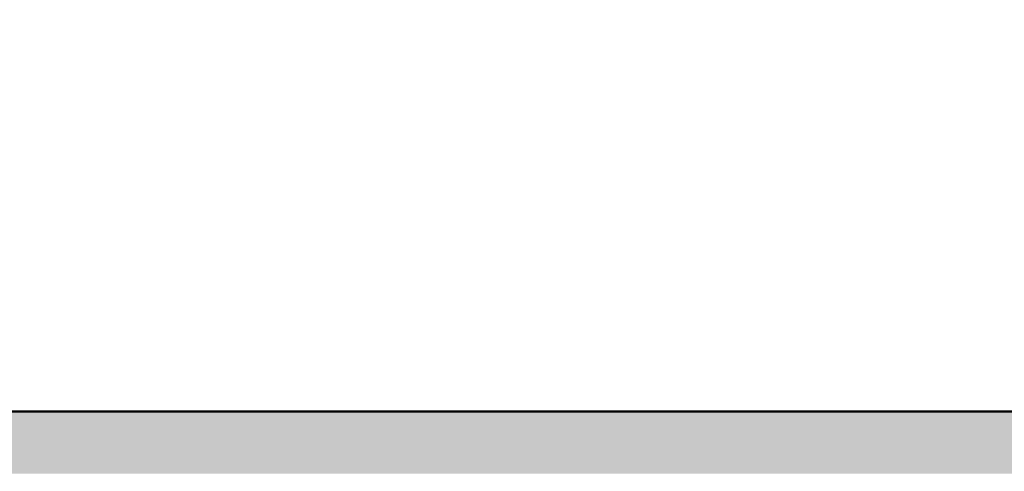
# Model space of a CAD drawing. Units: inches. Extents: x -7 to 1228, y -146 to 1091.
# Tile 13 of 88: x 105 to 200, y 487 to 531. Entities that reach past the tile are written whole.
import ezdxf

# ---------------------------------------------------------------- set-up
doc = ezdxf.new("R2010")
doc.units = ezdxf.units.IN
doc.layers.add('A-WALL', color=7, linetype='Continuous', lineweight=50)
doc.layers.add('A-WALL-PATT', color=251, linetype='Continuous', lineweight=13)

msp = doc.modelspace()

# ---------------------------------------------------------------- hatches: boundary and pattern name
at = {"layer": 'A-WALL-PATT'}
h = msp.add_hatch(color=256, dxfattribs=at)
h.dxf.hatch_style = 1
h.paths.add_polyline_path([(69, 568), (60, 568), (60, 493), (63.289, 493), (69, 493)])
h.paths.add_polyline_path([(69, 662.405), (60, 662.405), (60, 586), (69, 586)], flags=17)
h.paths.add_polyline_path([(69, 723), (184, 723), (184, 734), (179, 734), (179, 728), (69, 728), (69, 741.623), (60, 741.623), (60, 698.405), (69, 698.405)], flags=17)
h.paths.add_polyline_path([(69, 782), (231, 782), (231, 728), (231, 723), (231, 586), (236, 586), (236, 787), (69, 787), (69, 800.126), (60, 800.126), (60, 765.623), (69, 765.623)])
h.paths.add_polyline_path([(184, 842), (189, 842), (189, 848), (173, 848), (173, 842), (179, 842), (179, 787), (184, 787)])
h.paths.add_polyline_path([(118.22, 69), (69, 69), (69, 60), (118.22, 60)])
h.paths.add_polyline_path([(227, 69), (154.22, 69), (154.22, 60), (227, 60)])
h.paths.add_polyline_path([(236, 60), (232.711, 60), (227, 60), (227, 36), (236, 36)])
h.paths.add_polyline_path([(389, 60), (380, 60), (380, 36), (389, 36)])
h.paths.add_polyline_path([(384, 181), (380, 181), (380, 115), (380, 78), (384, 78)])
h.paths.add_polyline_path([(380, 115), (334.547, 115), (334.547, 109), (380, 109)])
h.paths.add_polyline_path([(274.547, 115), (236, 115), (236, 201), (232.711, 201), (231, 201), (231, 78), (236, 78), (236, 109), (274.547, 109)])
h.paths.add_polyline_path([(69, 123), (60, 123), (60, 78), (69, 78)])
h.paths.add_polyline_path([(69, 201), (60, 201), (60, 159), (69, 159)])
h.paths.add_polyline_path([(143, 219), (69, 219), (69, 213), (143, 213)], flags=17)
h.paths.add_polyline_path([(189, 219), (184, 219), (184, 274), (231, 274), (231, 219), (236, 219), (236, 279), (184, 279), (184, 297), (179, 297), (179, 279), (69, 279), (69, 290.912), (60, 290.912), (60, 262.179), (69, 262.179), (69, 274), (179, 274), (179, 219), (173, 219), (173, 213), (189, 213)])
h.paths.add_polyline_path([(69, 238.179), (60, 238.179), (60, 219), (69, 219)], flags=17)
h.paths.add_polyline_path([(69, 333), (60, 333), (60, 314.912), (69, 314.912), (69, 316.965)])
h.paths.add_polyline_path([(190, 338), (184, 338), (69, 338), (69, 333), (179, 333), (179, 327), (184, 327), (184, 333.021), (190, 333.046)])
h.paths.add_polyline_path([(69, 386.806), (60, 386.806), (60, 351), (69, 351)])
h.paths.add_polyline_path([(69, 475), (60, 475), (60, 422.806), (69, 422.806)])
h.paths.add_polyline_path([(236, 475), (231, 475), (231, 351.238), (236, 351.238)])
h.paths.add_polyline_path([(384, 475), (380, 475), (380, 362), (384, 362)])
h.paths.add_polyline_path([(547, 307), (439, 307), (439, 356), (445, 356), (445, 362), (433, 362), (433, 307), (380, 307), (380, 244), (380, 241), (384, 241), (384, 301), (433, 301), (433, 277), (439, 277), (439, 301), (547, 301)])
h.paths.add_polyline_path([(547, 241), (439, 241), (439, 247), (433, 247), (433, 235), (547, 235)])
h.paths.add_polyline_path([(450, 69), (440.286, 69), (424.889, 69), (389, 69), (389, 60), (450, 60)])
h.paths.add_polyline_path([(547, 69), (486, 69), (486, 60), (547, 60)])
h.paths.add_polyline_path([(556, 148.268), (547, 148.268), (547, 78), (556, 78)])
h.paths.add_polyline_path([(556, 223), (547, 223), (547, 195), (547, 184.268), (556, 184.268)])
h.paths.add_polyline_path([(556, 311.192), (547, 311.192), (547, 273.075), (556, 273.075)])
h.paths.add_polyline_path([(556, 344), (552.711, 344), (547, 344), (547, 335.192), (556, 335.192)])
h.paths.add_polyline_path([(556, 249.075), (547, 249.075), (547, 241), (556, 241)])
h.paths.add_polyline_path([(547, 362), (475, 362), (475, 356), (547, 356)], flags=0)
h.paths.add_polyline_path([(556, 399.621), (547, 399.621), (547, 362), (556, 362)])
h.paths.add_polyline_path([(556, 475), (547, 475), (547, 435.621), (556, 435.621)])
h.paths.add_polyline_path([(547, 493), (389, 493), (389, 487), (547, 487)])
h.paths.add_polyline_path([(380, 493), (278, 493), (278, 487), (380, 487)])
h.paths.add_polyline_path([(227, 493), (69, 493), (69, 487), (227, 487)])
h.paths.add_polyline_path([(643, 122.445), (634, 122.445), (634, 78), (643, 78)])
h.paths.add_polyline_path([(702.5, 69), (692.786, 69), (677.389, 69), (643, 69), (643, 60), (702.5, 60)])
h.paths.add_polyline_path([(798, 69), (738.5, 69), (738.5, 60), (798, 60)])
h.paths.add_polyline_path([(807, 60), (803.711, 60), (798, 60), (798, 36), (807, 36)])
h.paths.add_polyline_path([(807, 109), (846.751, 109), (846.751, 115), (807, 115), (807, 159), (802, 159), (802, 78), (807, 78)])
h.paths.add_polyline_path([(807, 201), (802, 201), (802, 195), (807, 195)])
h.paths.add_polyline_path([(643, 201), (634, 201), (634, 158.445), (643, 158.445)])
h.paths.add_polyline_path([(756, 225), (751, 225), (751, 219), (643, 219), (643, 213), (756, 213)])
h.paths.add_polyline_path([(643, 240.848), (634, 240.848), (634, 219), (643, 219)])
h.paths.add_polyline_path([(643, 274), (643, 288.629), (634, 288.629), (634, 264.848), (643, 264.848)])
h.paths.add_polyline_path([(802, 279), (756, 279), (756, 297), (751, 297), (751, 279), (643, 279), (643, 274), (751, 274), (751, 255), (756, 255), (756, 274), (802, 274)])
h.paths.add_polyline_path([(807, 333), (803.711, 333), (802, 333), (802, 279), (802, 274), (802, 219), (807, 219)])
h.paths.add_polyline_path([(956, 182), (951, 182), (951, 115), (906.751, 115), (906.751, 109), (951, 109), (951, 78), (956, 78)])
h.paths.add_polyline_path([(960, 60), (951, 60), (951, 36), (960, 36)])
h.paths.add_polyline_path([(1021, 69), (1005.781, 69), (960, 69), (960, 60), (1021, 60)])
h.paths.add_polyline_path([(956, 224), (951, 224), (951, 218), (956, 218)])
h.paths.add_polyline_path([(956, 302), (1004, 302), (1004, 278), (1010, 278), (1010, 302), (1118, 302), (1118, 290.809), (1127, 290.809), (1127, 326.968), (1118, 326.968), (1118, 320.966), (1118, 307), (1010, 307), (1010, 356), (1016, 356), (1016, 362), (1004, 362), (1004, 307), (951, 307), (951, 244), (951, 242), (954.289, 242), (956, 242)])
h.paths.add_polyline_path([(643, 333), (634, 333), (634, 312.629), (643, 312.629), (643, 316.965)])
h.paths.add_polyline_path([(756, 338), (643, 338), (643, 333), (751, 333), (751, 327), (756, 327)])
h.paths.add_polyline_path([(643, 388), (634, 388), (634, 351), (643, 351)])
h.paths.add_polyline_path([(807, 357), (802, 357), (802, 351), (807, 351)])
h.paths.add_polyline_path([(807, 475), (802, 475), (802, 393), (807, 393)])
h.paths.add_polyline_path([(643, 475), (634, 475), (634, 424), (643, 424)])
h.paths.add_polyline_path([(798, 493), (643, 493), (643, 487), (798, 487)])
h.paths.add_polyline_path([(634, 493), (556, 493), (556, 487), (634, 487)])
h.paths.add_polyline_path([(813, 493), (807, 493), (807, 487), (813, 487)])
h.paths.add_polyline_path([(951, 493), (849, 493), (849, 487), (951, 487)])
h.paths.add_polyline_path([(956, 484), (951, 484), (951, 374), (956, 374)])
h.paths.add_polyline_path([(1109, 493), (969, 493), (969, 487), (1109, 487)])
h.paths.add_polyline_path([(1127, 484), (1118, 484), (1118, 450.641), (1127, 450.641)])
h.paths.add_polyline_path([(1127, 414.641), (1118, 414.641), (1118, 365), (1127, 365)])
h.paths.add_polyline_path([(1109, 362), (1046, 362), (1046, 356), (1109, 356)], flags=17)
h.paths.add_polyline_path([(1127, 356), (1123.454, 356), (1118, 356), (1118, 350.968), (1127, 350.968)], flags=0)
h.paths.add_polyline_path([(1127, 266.809), (1118, 266.809), (1118, 262.361), (1118, 242), (1127, 242)], flags=17)
h.paths.add_polyline_path([(1118, 242), (1010, 242), (1010, 248), (1004, 248), (1004, 237), (1118, 237)])
h.paths.add_polyline_path([(1127, 224), (1118, 224), (1118, 170), (1127, 170)])
h.paths.add_polyline_path([(1127, 134), (1118, 134), (1118, 78), (1127, 78)])
h.paths.add_polyline_path([(1118, 69), (1057, 69), (1057, 60), (1118, 60)])
h.paths.add_polyline_path([(227, 571.546), (227, 574), (69, 574), (69, 568), (227, 568)])
h.paths.add_polyline_path([(380, 571.546), (380, 574), (278, 574), (278, 568), (380, 568)])
h.paths.add_polyline_path([(242, 574), (236, 574), (236, 568), (242, 568)])
h.paths.add_polyline_path([(547, 571.546), (547, 574), (389, 574), (389, 568), (547, 568)])
h.paths.add_polyline_path([(384, 733), (380, 733), (380, 586), (384, 586)])
h.paths.add_polyline_path([(556, 646), (634, 646), (634, 655), (547, 655), (547, 586), (556, 586)])
h.paths.add_polyline_path([(634, 574), (556, 574), (556, 568), (634, 568)])
h.paths.add_polyline_path([(643, 655), (634, 655), (634, 586), (643, 586)])
h.paths.add_polyline_path([(798, 574), (643, 574), (643, 568), (798, 568)])
h.paths.add_polyline_path([(643, 663.854), (634, 663.854), (634, 655), (643, 655)])
h.paths.add_polyline_path([(556, 676.967), (547, 676.967), (547, 655), (556, 655)])
h.paths.add_polyline_path([(556, 733), (547, 733), (547, 712.967), (556, 712.967)])
h.paths.add_polyline_path([(643, 710), (634, 710), (634, 699.854), (643, 699.854)])
h.paths.add_polyline_path([(807, 668), (802, 668), (802, 586), (807, 586)])
h.paths.add_polyline_path([(951, 574), (849, 574), (849, 568), (951, 568)])
h.paths.add_polyline_path([(956, 691), (951, 691), (951, 577), (956, 577)])
h.paths.add_polyline_path([(1109, 574), (969, 574), (969, 568), (1109, 568)])
h.paths.add_polyline_path([(1127, 643.403), (1118, 643.403), (1118, 577), (1127, 577)])
h.paths.add_polyline_path([(1127, 568), (1123.454, 568), (1118, 568), (1118, 493), (1127, 493)])
h.paths.add_polyline_path([(1127, 733), (1118, 733), (1118, 679.403), (1127, 679.403)])
h.paths.add_polyline_path([(1127, 777.348), (1118, 777.348), (1118, 770.035), (1118, 751), (1127, 751)], flags=17)
h.paths.add_polyline_path([(1118, 751), (1010, 751), (1010, 757), (1004, 757), (1004, 745), (1118, 745)])
h.paths.add_polyline_path([(956, 811), (1004, 811), (1004, 787), (1010, 787), (1010, 811), (1017.874, 811), (1017.874, 811.627, -0.414214), (1018.247, 812), (1031.978, 812, -0.414214), (1032.351, 811.627), (1032.351, 811), (1118, 811), (1118, 801.348), (1127, 801.348), (1127, 834.685), (1118, 834.685), (1118, 830.238), (1118, 817), (1010, 817), (1010, 866), (1016, 866), (1016, 872), (1004, 872), (1004, 817), (956, 817), (956, 866), (951, 866), (951, 751), (954.289, 751), (956, 751)])
h.paths.add_polyline_path([(1118, 872), (1046, 872), (1046, 866), (1118, 866)], flags=17)
h.paths.add_polyline_path([(1127, 924.711), (1118, 924.711), (1118, 884), (1127, 884)])
h.paths.add_polyline_path([(1127, 866), (1123.711, 866), (1118, 866), (1118, 858.685), (1127, 858.685)], flags=17)
h.paths.add_polyline_path([(956, 983), (951, 983), (951, 952), (807, 952), (807, 983), (802, 983), (802, 902), (807, 902), (807, 946), (951, 946), (951, 884), (956, 884)])
h.paths.add_polyline_path([(807, 842), (802, 842), (802, 787), (756, 787), (756, 806), (751, 806), (751, 787), (643, 787), (643, 782), (751, 782), (751, 764), (756, 764), (756, 782), (802, 782), (802, 728), (807, 728)])
h.paths.add_polyline_path([(756, 848), (643, 848), (643, 842), (751, 842), (751, 836), (756, 836)])
h.paths.add_polyline_path([(756, 734), (751, 734), (751, 728), (643, 728), (643, 723), (756, 723)])
h.paths.add_polyline_path([(643, 749.791), (634, 749.791), (634, 728), (637.289, 728), (643, 728)])
h.paths.add_polyline_path([(643, 805.405), (634, 805.405), (634, 773.791), (643, 773.791)])
h.paths.add_polyline_path([(643, 896.663), (634, 896.663), (634, 860), (637.289, 860), (643, 860)])
h.paths.add_polyline_path([(643, 842), (634, 842), (634, 829.405), (643, 829.405)])
h.paths.add_polyline_path([(643, 983), (634, 983), (634, 932.663), (643, 932.663)])
h.paths.add_polyline_path([(1127, 983), (1118, 983), (1118, 960.711), (1127, 960.711)])
h.paths.add_polyline_path([(1118, 1001), (1077.525, 1001), (1077.525, 992), (1118, 992)])
h.paths.add_polyline_path([(1041.525, 1001), (960, 1001), (960, 992), (1041.525, 992)])
h.paths.add_polyline_path([(960, 1025), (951, 1025), (951, 1001), (954.289, 1001), (960, 1001)])
h.paths.add_polyline_path([(807, 1025), (798, 1025), (798, 1001), (807, 1001)])
h.paths.add_polyline_path([(798, 1001), (738.5, 1001), (738.5, 992), (798, 992)])
h.paths.add_polyline_path([(702.5, 1001), (643, 1001), (643, 992), (702.5, 992)])
h.paths.add_polyline_path([(547, 1001), (499.113, 1001), (499.113, 992), (547, 992)])
h.paths.add_polyline_path([(463.113, 1001), (389, 1001), (389, 992), (463.113, 992)])
h.paths.add_polyline_path([(389, 1025), (380, 1025), (380, 1022), (380, 1001), (383.289, 1001), (389, 1001)])
h.paths.add_polyline_path([(236, 1025), (227, 1025), (227, 1001), (236, 1001)])
h.paths.add_polyline_path([(236, 983), (231, 983), (231, 860), (236, 860)])
h.paths.add_polyline_path([(274.547, 952), (236, 952), (236, 946), (274.547, 946)])
h.paths.add_polyline_path([(380, 952), (334.547, 952), (334.547, 946), (380, 946)])
h.paths.add_polyline_path([(384, 983), (380, 983), (380, 884), (383.289, 884), (384, 884)])
h.paths.add_polyline_path([(227, 1001), (155.012, 1001), (155.012, 992), (162.875, 992), (227, 992)])
h.paths.add_polyline_path([(119.012, 1001), (69, 1001), (69, 992), (119.012, 992)])
h.paths.add_polyline_path([(69, 983), (60, 983), (60, 922.987), (69, 922.987)])
h.paths.add_polyline_path([(69, 886.987), (60, 886.987), (60, 860), (63.289, 860), (69, 860)])
h.paths.add_polyline_path([(143, 848), (69, 848), (69, 842), (143, 842)])

# ---------------------------------------------------------------- linework, layer by layer
at = {"layer": 'A-WALL'}
msp.add_line((231, 493), (60, 493), dxfattribs=at)

doc.saveas('drawing.dxf')
